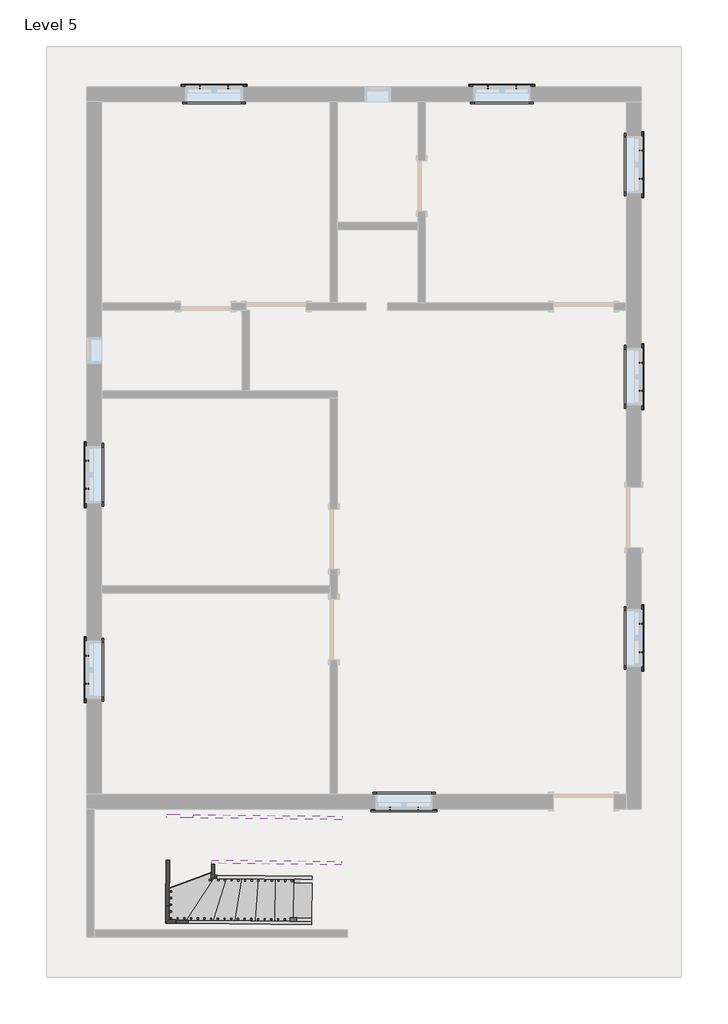
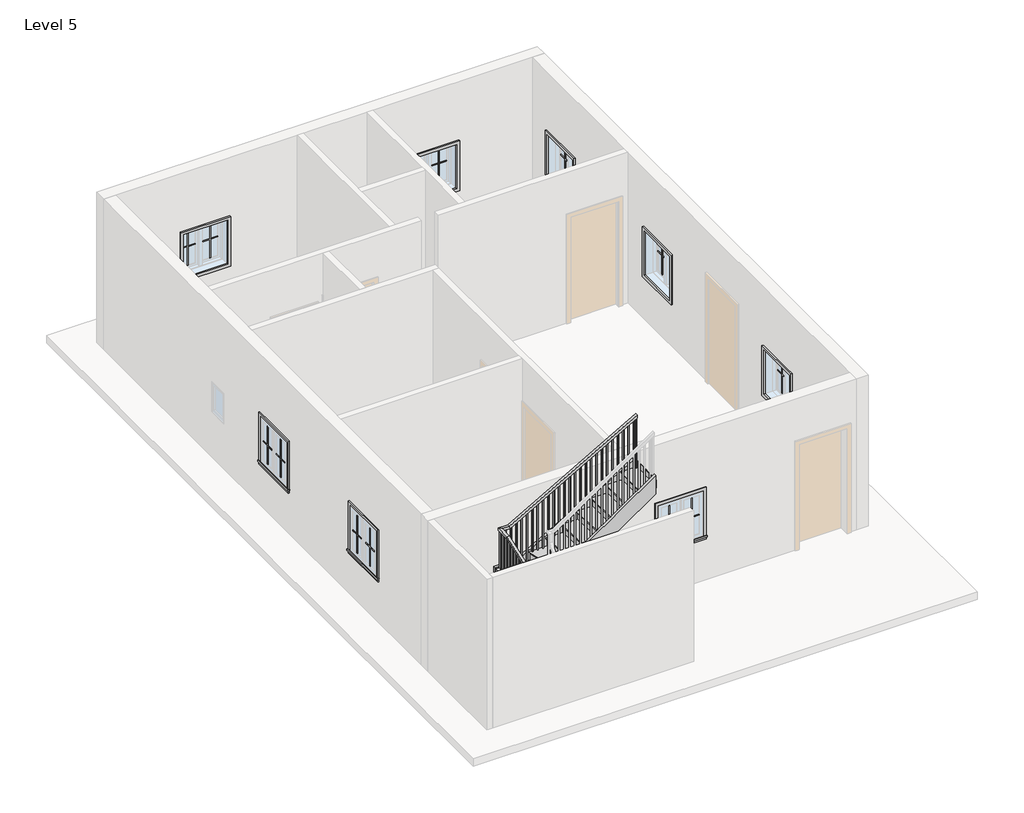
# One storey, part 2 of 2: 32 proxies, 9 members, 1 railing, 1 stair flight.
"""IFC4 building model written with IfcOpenShell, lengths in millimetres."""

from ifc_helpers import new_model, si_unit, frame, origin, place, context, project, spatial, polyline, outline, extrude, faceted_brep, transform, mapped, element, save
from components import muntin_pattern_2x2_muntin_pattern_2x2_b3fe6957, muntin_pattern_2x2_muntin_pattern_2x2_3e0ecaf2, trim_window_exterior_flat_with_sill_41619996, trim_window_interior_flat_picture_frame_51c85655, stair_flight_e36c3716

model = new_model("IFC4")

# Units and contexts
model_context = context("Model", 3, world=origin())
ifc_project = project(units=[si_unit("LENGTHUNIT", "METRE", prefix="MILLI")], contexts=[model_context])

# Site, building, storey
site = spatial("IfcSite", under=ifc_project)
building = spatial("IfcBuilding", under=site)
storey = spatial("IfcBuildingStorey", under=building, Name="Level 5", Elevation=9601.2)

# Proxies
placement = place(None, origin())
muntin_pattern_2x2_muntin_pattern_2x2_shape = muntin_pattern_2x2_muntin_pattern_2x2_b3fe6957(model_context)
element("IfcBuildingElementProxy", 1, Name="Muntin Pattern_2x2 : Muntin Pattern_2x2", ObjectType="Muntin Pattern_2x2 : Muntin Pattern_2x2", at=placement, inside=storey, context=model_context, shape_type="MappedRepresentation", body=[
    mapped(muntin_pattern_2x2_muntin_pattern_2x2_shape, transform((-3662.5622832, 7052.6782079, 10585.45), x_axis=(1.0, 0.0, 0.0), y_axis=(0.0, 1.0, 0.0), z_axis=(0.0, 0.0, 1.0))),
])
element("IfcBuildingElementProxy", 2, Name="Muntin Pattern_2x2 : Muntin Pattern_2x2", ObjectType="Muntin Pattern_2x2 : Muntin Pattern_2x2", at=placement, inside=storey, context=model_context, shape_type="MappedRepresentation", body=[
    mapped(muntin_pattern_2x2_muntin_pattern_2x2_shape, transform((709.4127168, 7052.6782079, 10585.45), x_axis=(1.0, 0.0, 0.0), y_axis=(0.0, 1.0, 0.0), z_axis=(0.0, 0.0, 1.0))),
])
element("IfcBuildingElementProxy", 3, Name="Muntin Pattern_2x2 : Muntin Pattern_2x2", ObjectType="Muntin Pattern_2x2 : Muntin Pattern_2x2", at=placement, inside=storey, context=model_context, shape_type="MappedRepresentation", body=[
    mapped(muntin_pattern_2x2_muntin_pattern_2x2_shape, transform((3028.7502168, 6095.4157079, 10585.45), x_axis=(0.0, -1.0, 0.0), y_axis=(1.0, 0.0, 0.0), z_axis=(0.0, 0.0, 1.0))),
])
element("IfcBuildingElementProxy", 4, Name="Muntin Pattern_2x2 : Muntin Pattern_2x2", ObjectType="Muntin Pattern_2x2 : Muntin Pattern_2x2", at=placement, inside=storey, context=model_context, shape_type="MappedRepresentation", body=[
    mapped(muntin_pattern_2x2_muntin_pattern_2x2_shape, transform((3028.7502168, 2875.9657079, 10585.45), x_axis=(0.0, -1.0, 0.0), y_axis=(1.0, 0.0, 0.0), z_axis=(0.0, 0.0, 1.0))),
])
element("IfcBuildingElementProxy", 5, Name="Muntin Pattern_2x2 : Muntin Pattern_2x2", ObjectType="Muntin Pattern_2x2 : Muntin Pattern_2x2", at=placement, inside=storey, context=model_context, shape_type="MappedRepresentation", body=[
    mapped(muntin_pattern_2x2_muntin_pattern_2x2_shape, transform((3028.7502168, -1086.4342921, 10585.45), x_axis=(0.0, -1.0, 0.0), y_axis=(1.0, 0.0, 0.0), z_axis=(0.0, 0.0, 1.0))),
])
element("IfcBuildingElementProxy", 6, Name="Muntin Pattern_2x2 : Muntin Pattern_2x2", ObjectType="Muntin Pattern_2x2 : Muntin Pattern_2x2", at=placement, inside=storey, context=model_context, shape_type="MappedRepresentation", body=[
    mapped(muntin_pattern_2x2_muntin_pattern_2x2_shape, transform((-5372.2997832, 961.4407079, 10585.45), x_axis=(0.0, 1.0, 0.0), y_axis=(-1.0, 0.0, 0.0), z_axis=(0.0, 0.0, 1.0))),
])
element("IfcBuildingElementProxy", 7, Name="Muntin Pattern_2x2 : Muntin Pattern_2x2", ObjectType="Muntin Pattern_2x2 : Muntin Pattern_2x2", at=placement, inside=storey, context=model_context, shape_type="MappedRepresentation", body=[
    mapped(muntin_pattern_2x2_muntin_pattern_2x2_shape, transform((-5372.2997832, -1997.6592921, 10585.45), x_axis=(0.0, 1.0, 0.0), y_axis=(-1.0, 0.0, 0.0), z_axis=(0.0, 0.0, 1.0))),
])
element("IfcBuildingElementProxy", 8, Name="Muntin Pattern_2x2 : Muntin Pattern_2x2", ObjectType="Muntin Pattern_2x2 : Muntin Pattern_2x2", at=placement, inside=storey, context=model_context, shape_type="MappedRepresentation", body=[
    mapped(muntin_pattern_2x2_muntin_pattern_2x2_shape, transform((-347.8622832, -3888.3717921, 10585.45), x_axis=(-1.0, 0.0, 0.0), y_axis=(0.0, -1.0, 0.0), z_axis=(0.0, 0.0, 1.0))),
])
muntin_pattern_2x2_muntin_pattern_2x2_2_shape = muntin_pattern_2x2_muntin_pattern_2x2_3e0ecaf2(model_context)
element("IfcBuildingElementProxy", 9, Name="Muntin Pattern_2x2 : Muntin Pattern_2x2", ObjectType="Muntin Pattern_2x2 : Muntin Pattern_2x2", at=placement, inside=storey, context=model_context, shape_type="MappedRepresentation", body=[
    mapped(muntin_pattern_2x2_muntin_pattern_2x2_2_shape, transform((-3233.9372832, 7052.6782079, 10585.45), x_axis=(-1.0, 0.0, 0.0), y_axis=(0.0, -1.0, 0.0), z_axis=(0.0, 0.0, 1.0))),
])
element("IfcBuildingElementProxy", 10, Name="Muntin Pattern_2x2 : Muntin Pattern_2x2", ObjectType="Muntin Pattern_2x2 : Muntin Pattern_2x2", at=placement, inside=storey, context=model_context, shape_type="MappedRepresentation", body=[
    mapped(muntin_pattern_2x2_muntin_pattern_2x2_2_shape, transform((1138.0377168, 7052.6782079, 10585.45), x_axis=(-1.0, 0.0, 0.0), y_axis=(0.0, -1.0, 0.0), z_axis=(0.0, 0.0, 1.0))),
])
element("IfcBuildingElementProxy", 11, Name="Muntin Pattern_2x2 : Muntin Pattern_2x2", ObjectType="Muntin Pattern_2x2 : Muntin Pattern_2x2", at=placement, inside=storey, context=model_context, shape_type="MappedRepresentation", body=[
    mapped(muntin_pattern_2x2_muntin_pattern_2x2_2_shape, transform((3028.7502168, 5666.7907079, 10585.45), x_axis=(0.0, 1.0, 0.0), y_axis=(-1.0, 0.0, 0.0), z_axis=(0.0, 0.0, 1.0))),
])
element("IfcBuildingElementProxy", 12, Name="Muntin Pattern_2x2 : Muntin Pattern_2x2", ObjectType="Muntin Pattern_2x2 : Muntin Pattern_2x2", at=placement, inside=storey, context=model_context, shape_type="MappedRepresentation", body=[
    mapped(muntin_pattern_2x2_muntin_pattern_2x2_2_shape, transform((3028.7502168, 2447.3407079, 10585.45), x_axis=(0.0, 1.0, 0.0), y_axis=(-1.0, 0.0, 0.0), z_axis=(0.0, 0.0, 1.0))),
])
element("IfcBuildingElementProxy", 13, Name="Muntin Pattern_2x2 : Muntin Pattern_2x2", ObjectType="Muntin Pattern_2x2 : Muntin Pattern_2x2", at=placement, inside=storey, context=model_context, shape_type="MappedRepresentation", body=[
    mapped(muntin_pattern_2x2_muntin_pattern_2x2_2_shape, transform((3028.7502168, -1515.0592921, 10585.45), x_axis=(0.0, 1.0, 0.0), y_axis=(-1.0, 0.0, 0.0), z_axis=(0.0, 0.0, 1.0))),
])
element("IfcBuildingElementProxy", 14, Name="Muntin Pattern_2x2 : Muntin Pattern_2x2", ObjectType="Muntin Pattern_2x2 : Muntin Pattern_2x2", at=placement, inside=storey, context=model_context, shape_type="MappedRepresentation", body=[
    mapped(muntin_pattern_2x2_muntin_pattern_2x2_2_shape, transform((-5372.2997832, 1390.0657079, 10585.45), x_axis=(0.0, -1.0, 0.0), y_axis=(1.0, 0.0, 0.0), z_axis=(0.0, 0.0, 1.0))),
])
element("IfcBuildingElementProxy", 15, Name="Muntin Pattern_2x2 : Muntin Pattern_2x2", ObjectType="Muntin Pattern_2x2 : Muntin Pattern_2x2", at=placement, inside=storey, context=model_context, shape_type="MappedRepresentation", body=[
    mapped(muntin_pattern_2x2_muntin_pattern_2x2_2_shape, transform((-5372.2997832, -1569.0342921, 10585.45), x_axis=(0.0, -1.0, 0.0), y_axis=(1.0, 0.0, 0.0), z_axis=(0.0, 0.0, 1.0))),
])
element("IfcBuildingElementProxy", 16, Name="Muntin Pattern_2x2 : Muntin Pattern_2x2", ObjectType="Muntin Pattern_2x2 : Muntin Pattern_2x2", at=placement, inside=storey, context=model_context, shape_type="MappedRepresentation", body=[
    mapped(muntin_pattern_2x2_muntin_pattern_2x2_2_shape, transform((-776.4872832, -3888.3717921, 10585.45), x_axis=(1.0, 0.0, 0.0), y_axis=(0.0, 1.0, 0.0), z_axis=(0.0, 0.0, 1.0))),
])
trim_window_exterior_flat_with_sill_shape = trim_window_exterior_flat_with_sill_41619996(model_context)
element("IfcBuildingElementProxy", 17, Name="Trim-Window-Exterior-Flat : with Sill", ObjectType="Trim-Window-Exterior-Flat : with Sill", at=placement, inside=storey, context=model_context, shape_type="MappedRepresentation", body=[
    mapped(trim_window_exterior_flat_with_sill_shape, transform((-3448.2497832, 7062.2032079, 11430.0), x_axis=(-1.0, 0.0, 0.0), y_axis=(0.0, 0.0, 1.0), z_axis=(0.0, 1.0, 0.0))),
])
element("IfcBuildingElementProxy", 18, Name="Trim-Window-Exterior-Flat : with Sill", ObjectType="Trim-Window-Exterior-Flat : with Sill", at=placement, inside=storey, context=model_context, shape_type="MappedRepresentation", body=[
    mapped(trim_window_exterior_flat_with_sill_shape, transform((923.7252168, 7062.2032079, 11430.0), x_axis=(-1.0, 0.0, 0.0), y_axis=(0.0, 0.0, 1.0), z_axis=(0.0, 1.0, 0.0))),
])
element("IfcBuildingElementProxy", 19, Name="Trim-Window-Exterior-Flat : with Sill", ObjectType="Trim-Window-Exterior-Flat : with Sill", at=placement, inside=storey, context=model_context, shape_type="MappedRepresentation", body=[
    mapped(trim_window_exterior_flat_with_sill_shape, transform((3038.2752168, 5881.1032079, 11430.0), x_axis=(0.0, 1.0, 0.0), y_axis=(0.0, 0.0, 1.0), z_axis=(1.0, 0.0, 0.0))),
])
element("IfcBuildingElementProxy", 20, Name="Trim-Window-Exterior-Flat : with Sill", ObjectType="Trim-Window-Exterior-Flat : with Sill", at=placement, inside=storey, context=model_context, shape_type="MappedRepresentation", body=[
    mapped(trim_window_exterior_flat_with_sill_shape, transform((3038.2752168, 2661.6532079, 11430.0), x_axis=(0.0, 1.0, 0.0), y_axis=(0.0, 0.0, 1.0), z_axis=(1.0, 0.0, 0.0))),
])
element("IfcBuildingElementProxy", 21, Name="Trim-Window-Exterior-Flat : with Sill", ObjectType="Trim-Window-Exterior-Flat : with Sill", at=placement, inside=storey, context=model_context, shape_type="MappedRepresentation", body=[
    mapped(trim_window_exterior_flat_with_sill_shape, transform((3038.2752168, -1300.7467921, 11430.0), x_axis=(0.0, 1.0, 0.0), y_axis=(0.0, 0.0, 1.0), z_axis=(1.0, 0.0, 0.0))),
])
element("IfcBuildingElementProxy", 22, Name="Trim-Window-Exterior-Flat : with Sill", ObjectType="Trim-Window-Exterior-Flat : with Sill", at=placement, inside=storey, context=model_context, shape_type="MappedRepresentation", body=[
    mapped(trim_window_exterior_flat_with_sill_shape, transform((-5381.8247832, 1175.7532079, 11430.0), x_axis=(0.0, -1.0, 0.0), y_axis=(0.0, 0.0, 1.0), z_axis=(-1.0, 0.0, 0.0))),
])
element("IfcBuildingElementProxy", 23, Name="Trim-Window-Exterior-Flat : with Sill", ObjectType="Trim-Window-Exterior-Flat : with Sill", at=placement, inside=storey, context=model_context, shape_type="MappedRepresentation", body=[
    mapped(trim_window_exterior_flat_with_sill_shape, transform((-5381.8247832, -1783.3467921, 11430.0), x_axis=(0.0, -1.0, 0.0), y_axis=(0.0, 0.0, 1.0), z_axis=(-1.0, 0.0, 0.0))),
])
element("IfcBuildingElementProxy", 24, Name="Trim-Window-Exterior-Flat : with Sill", ObjectType="Trim-Window-Exterior-Flat : with Sill", at=placement, inside=storey, context=model_context, shape_type="MappedRepresentation", body=[
    mapped(trim_window_exterior_flat_with_sill_shape, transform((-562.1747832, -3897.8967921, 11430.0), x_axis=(1.0, 0.0, 0.0), y_axis=(0.0, 0.0, 1.0), z_axis=(0.0, -1.0, 0.0))),
])
trim_window_interior_flat_picture_frame_shape = trim_window_interior_flat_picture_frame_51c85655(model_context)
element("IfcBuildingElementProxy", 25, Name="Trim-Window-Interior-Flat : Picture Frame", ObjectType="Trim-Window-Interior-Flat : Picture Frame", at=placement, inside=storey, context=model_context, shape_type="MappedRepresentation", body=[
    mapped(trim_window_interior_flat_picture_frame_shape, transform((-3448.2497832, 6833.6032079, 11430.0), x_axis=(1.0, 0.0, 0.0), y_axis=(0.0, 0.0, 1.0), z_axis=(0.0, -1.0, 0.0))),
])
element("IfcBuildingElementProxy", 26, Name="Trim-Window-Interior-Flat : Picture Frame", ObjectType="Trim-Window-Interior-Flat : Picture Frame", at=placement, inside=storey, context=model_context, shape_type="MappedRepresentation", body=[
    mapped(trim_window_interior_flat_picture_frame_shape, transform((923.7252168, 6833.6032079, 11430.0), x_axis=(1.0, 0.0, 0.0), y_axis=(0.0, 0.0, 1.0), z_axis=(0.0, -1.0, 0.0))),
])
element("IfcBuildingElementProxy", 27, Name="Trim-Window-Interior-Flat : Picture Frame", ObjectType="Trim-Window-Interior-Flat : Picture Frame", at=placement, inside=storey, context=model_context, shape_type="MappedRepresentation", body=[
    mapped(trim_window_interior_flat_picture_frame_shape, transform((2809.6752168, 5881.1032079, 11430.0), x_axis=(0.0, -1.0, 0.0), y_axis=(0.0, 0.0, 1.0), z_axis=(-1.0, 0.0, 0.0))),
])
element("IfcBuildingElementProxy", 28, Name="Trim-Window-Interior-Flat : Picture Frame", ObjectType="Trim-Window-Interior-Flat : Picture Frame", at=placement, inside=storey, context=model_context, shape_type="MappedRepresentation", body=[
    mapped(trim_window_interior_flat_picture_frame_shape, transform((2809.6752168, 2661.6532079, 11430.0), x_axis=(0.0, -1.0, 0.0), y_axis=(0.0, 0.0, 1.0), z_axis=(-1.0, 0.0, 0.0))),
])
element("IfcBuildingElementProxy", 29, Name="Trim-Window-Interior-Flat : Picture Frame", ObjectType="Trim-Window-Interior-Flat : Picture Frame", at=placement, inside=storey, context=model_context, shape_type="MappedRepresentation", body=[
    mapped(trim_window_interior_flat_picture_frame_shape, transform((2809.6752168, -1300.7467921, 11430.0), x_axis=(0.0, -1.0, 0.0), y_axis=(0.0, 0.0, 1.0), z_axis=(-1.0, 0.0, 0.0))),
])
element("IfcBuildingElementProxy", 30, Name="Trim-Window-Interior-Flat : Picture Frame", ObjectType="Trim-Window-Interior-Flat : Picture Frame", at=placement, inside=storey, context=model_context, shape_type="MappedRepresentation", body=[
    mapped(trim_window_interior_flat_picture_frame_shape, transform((-5153.2247832, 1175.7532079, 11430.0), x_axis=(0.0, 1.0, 0.0), y_axis=(0.0, 0.0, 1.0), z_axis=(1.0, 0.0, 0.0))),
])
element("IfcBuildingElementProxy", 31, Name="Trim-Window-Interior-Flat : Picture Frame", ObjectType="Trim-Window-Interior-Flat : Picture Frame", at=placement, inside=storey, context=model_context, shape_type="MappedRepresentation", body=[
    mapped(trim_window_interior_flat_picture_frame_shape, transform((-5153.2247832, -1783.3467921, 11430.0), x_axis=(0.0, 1.0, 0.0), y_axis=(0.0, 0.0, 1.0), z_axis=(1.0, 0.0, 0.0))),
])
element("IfcBuildingElementProxy", 32, Name="Trim-Window-Interior-Flat : Picture Frame", ObjectType="Trim-Window-Interior-Flat : Picture Frame", at=placement, inside=storey, context=model_context, shape_type="MappedRepresentation", body=[
    mapped(trim_window_interior_flat_picture_frame_shape, transform((-562.1747832, -3669.2967921, 11430.0), x_axis=(-1.0, 0.0, 0.0), y_axis=(0.0, 0.0, 1.0), z_axis=(0.0, 1.0, 0.0))),
])

# Members
element("IfcMember", 33, ObjectType="Stringer - 2\" Width", at=placement, inside=storey, context=model_context, shape_type="SweptSolid", body=[
    extrude(outline(polyline([(-105.6395382, -202.4353776), (0.0, 0.0), (2328.2458671, 0.0), (2169.1880402, -304.8), (90.52017, -304.8), (-105.6395382, -202.4353776)])), frame((-1968.9977307, -5651.1672049, 9829.5413982), z_axis=(0.01073603161956521, 0.9999423671517593, 0.0), x_axis=(-0.8864958884204138, 0.009517996437940355, 0.46263857119517027)), (0.0, 0.0, 1.0), 50.8),
])
element("IfcMember", 34, ObjectType="Stringer - 2\" Width", at=placement, inside=storey, context=model_context, shape_type="SweptSolid", body=[
    extrude(outline(polyline([(-4032.4327287, -5578.2098967), (-4032.9781191, -5629.006969), (-4182.4018504, -5627.4026586), (-4131.0593878, -5577.1509768), (-4032.4327287, -5578.2098967)])), frame((0.0, 0.0, 10562.8719334), z_axis=(0.0, 0.0, 1.0), x_axis=(1.0, 0.0, 0.0)), (0.0, 0.0, 1.0), 343.8058061),
])
element("IfcMember", 35, ObjectType="Stringer - 2\" Width", at=placement, inside=storey, context=model_context, shape_type="SweptSolid", body=[
    extrude(outline(polyline([(-4131.0593878, -5577.1509768), (-4182.4018504, -5627.4026586), (-4179.6442274, -5370.5606366), (-4128.8471552, -5371.106027), (-4131.0593878, -5577.1509768)])), frame((0.0, 0.0, 10562.8719334), z_axis=(0.0, 0.0, 1.0), x_axis=(1.0, 0.0, 0.0)), (0.0, 0.0, 1.0), 343.8058061),
])
element("IfcMember", 36, ObjectType="Stringer - 2\" Width", at=placement, inside=storey, context=model_context, shape_type="SweptSolid", body=[
    extrude(outline(polyline([(110.9788635, -325.4014815), (0.0, 0.0), (1419.3210826, 0.0), (1526.5904374, -314.5248191), (1494.6989405, -325.4014816), (110.9788635, -325.4014815)])), frame((-4128.8471552, -5371.106027, 10562.8719334), z_axis=(-0.9999423671517593, 0.010736031619565298, 0.0), x_axis=(0.010161319362697869, 0.946414289466532, 0.3227951986668461)), (0.0, 0.0, 1.0), 50.8),
])
element("IfcMember", 37, ObjectType="Stringer - 2\" Width", at=placement, inside=storey, context=model_context, shape_type="SweptSolid", body=[
    extrude(outline(polyline([(-4165.2220526, -4027.2948827), (-4164.6766622, -3976.4978105), (-3763.6581151, -3980.8034064), (-3764.2035055, -4031.6004787), (-4165.2220526, -4027.2948827)])), frame((0.0, 0.0, 11031.2968076), z_axis=(0.0, 0.0, 1.0), x_axis=(1.0, 0.0, 0.0)), (0.0, 0.0, 1.0), 322.0391291),
])
element("IfcMember", 38, ObjectType="Stringer - 2\" Width", at=placement, inside=storey, context=model_context, shape_type="SweptSolid", body=[
    extrude(outline(polyline([(-111.9640108, -160.4153284), (0.0, 0.0), (1801.1015507, 0.0), (1588.362339, -304.8), (94.9016984, -304.8), (-111.9640108, -160.4153284)])), frame((-1961.6349602, -4965.4067295, 9796.8246848), z_axis=(0.010736031619565371, 0.9999423671517593, 0.0), x_axis=(-0.8199685195580257, 0.008803715336213096, 0.5723409137307053)), (0.0, 0.0, 1.0), 50.8),
])
element("IfcMember", 39, ObjectType="Stringer - 2\" Width", at=placement, inside=storey, context=model_context, shape_type="SweptSolid", body=[
    extrude(outline(polyline([(451.3522078, -304.8), (7.554265, -5.1014262), (10.999279, 0.0), (408.4725128, 0.0), (831.8908901, -285.9361695), (819.1520678, -304.8), (451.3522078, -304.8)])), frame((-3438.4815323, -4949.5503441, 10482.3097108), z_axis=(-0.9999423671517593, 0.010736031619565902, 0.0), x_axis=(0.00600837694393381, 0.559613726649973, 0.8287317879455506)), (0.0, 0.0, 1.0), 50.8),
])
element("IfcMember", 40, ObjectType="Stringer - 2\" Width", at=placement, inside=storey, context=model_context, shape_type="SweptSolid", body=[
    extrude(outline(polyline([(215.732707, -304.8), (0.0, 0.0), (2421.4097535, 0.0), (2637.1424605, -304.8), (215.732707, -304.8)])), frame((-3486.8243477, -4720.4181286, 10958.3256311), z_axis=(0.010736031619565212, 0.9999423671517593, 0.0), x_axis=(0.8161886957592971, -0.008763132689499912, 0.5777189804915569)), (0.0, 0.0, 1.0), 50.8),
])
element("IfcMember", 41, ObjectType="Stringer - 2\" Width", at=placement, inside=storey, context=model_context, shape_type="SweptSolid", body=[
    extrude(outline(polyline([(161.6856691, -278.5084291), (0.0, 0.0), (2614.6236412, 0.0), (2776.3093103, -278.508429), (161.6856691, -278.5084291)])), frame((-3764.2035055, -4031.6004787, 11031.2968076), z_axis=(0.01073603161956531, 0.9999423671517593, 0.0), x_axis=(0.8647780740833296, -0.009284819857879231, 0.5020683964410966)), (0.0, 0.0, 1.0), 50.8),
])

# Railing
element("IfcRailing", 42, ObjectType="Handrail - Rectangular", at=placement, inside=storey, context=model_context, shape_type="SolidModel", body=[
    faceted_brep([(-1968.4523403, -5600.3701326, 10684.9333333), (-1968.4523403, -5600.3701326, 10627.3388957), (-1967.9069499, -5549.5730604, 10627.3388957), (-1967.9069499, -5549.5730604, 10684.9333333), (-4009.5042766, -5578.4560715, 11775.3579081), (-4022.2220752, -5578.319525, 11724.5579081), (-4021.6766848, -5527.5224527, 11724.5579081), (-4008.9588862, -5527.6589993, 11775.3579081), (-4131.0593878, -5577.1509768, 11775.3579081), (-4131.0593878, -5577.1509768, 11724.5579081), (-4079.7169251, -5526.8992949, 11724.5579081), (-4079.7169251, -5526.8992949, 11775.3579081), (-4129.1695675, -5401.1351667, 11775.3579081), (-4129.079122, -5392.7111679, 11724.5579081), (-4078.2820498, -5393.2565584, 11724.5579081), (-4078.3724953, -5401.6805571, 11775.3579081), (-4117.5603361, -4319.8639155, 12144.1490097), (-4117.4698906, -4311.4399167, 12093.3490097), (-4066.6728183, -4311.9853071, 12093.3490097), (-4066.7632639, -4320.4093059, 12144.1490097), (-4114.4249804, -4027.8402731, 12144.1490097), (-4114.4249804, -4027.8402731, 12093.3490097), (-4064.1732985, -4079.1827358, 12093.3490097), (-4064.1732985, -4079.1827358, 12144.1490097), (-3933.3337165, -4029.7845867, 12144.1490097), (-3919.5861077, -4029.93219, 12093.3490097), (-3920.1314981, -4080.7292622, 12093.3490097), (-3933.8791069, -4080.581659, 12144.1490097), (-1503.1343086, -4055.8767882, 13563.6), (-1503.679699, -4106.6738604, 13563.6), (-1503.679699, -4106.6738604, 13504.7701828), (-1503.1343086, -4055.8767882, 13504.7701828)], [[[0, 1, 2, 3]], [[1, 0, 4, 5]], [[2, 1, 5, 6]], [[3, 2, 6, 7]], [[0, 3, 7, 4]], [[5, 4, 8, 9]], [[6, 5, 9, 10]], [[7, 6, 10, 11]], [[4, 7, 11, 8]], [[9, 8, 12, 13]], [[10, 9, 13, 14]], [[11, 10, 14, 15]], [[8, 11, 15, 12]], [[13, 12, 16, 17]], [[14, 13, 17, 18]], [[15, 14, 18, 19]], [[12, 15, 19, 16]], [[17, 16, 20, 21]], [[18, 17, 21, 22]], [[19, 18, 22, 23]], [[16, 19, 23, 20]], [[21, 20, 24, 25]], [[22, 21, 25, 26]], [[23, 22, 26, 27]], [[20, 23, 27, 24]], [[28, 29, 30, 31]], [[25, 24, 28, 31]], [[26, 25, 31, 30]], [[27, 26, 30, 29]], [[24, 27, 29, 28]]]),
    extrude(outline(polyline([(234.1631202, 19.05), (1226.6129544, 19.05), (1226.6129544, 0.0), (223.0368797, 0.0), (234.1631202, 19.05)])), frame((-1540.0233365, -4090.4077365, 13706.4796211), z_axis=(0.010736031619565153, 0.9999423671517594, 0.0), x_axis=(0.0, 0.0, -1.0)), (0.0, 0.0, 1.0), 19.05),
    extrude(outline(polyline([(234.1631202, 19.05), (1167.2730054, 19.05), (1167.2730054, 0.0), (223.0368798, 0.0), (234.1631202, 19.05)])), frame((-1641.617481, -4089.3169557, 13647.1396721), z_axis=(0.010736031619565153, 0.9999423671517594, 0.0), x_axis=(0.0, 0.0, -1.0)), (0.0, 0.0, 1.0), 19.05),
    extrude(outline(polyline([(234.1631202, 19.05), (1107.9330563, 19.05), (1107.9330563, 0.0), (223.0368797, 0.0), (234.1631202, 19.05)])), frame((-1743.2116255, -4088.2261749, 13587.799723), z_axis=(0.010736031619565153, 0.9999423671517594, 0.0), x_axis=(0.0, 0.0, -1.0)), (0.0, 0.0, 1.0), 19.05),
    extrude(outline(polyline([(234.1631202, 19.05), (1217.9264407, 19.05), (1217.9264407, 0.0), (223.0368798, 0.0), (234.1631202, 19.05)])), frame((-1844.80577, -4087.1353941, 13528.459774), z_axis=(0.010736031619565153, 0.9999423671517594, 0.0), x_axis=(0.0, 0.0, -1.0)), (0.0, 0.0, 1.0), 19.05),
    extrude(outline(polyline([(234.1631203, 19.05), (1158.5864917, 19.05), (1158.5864917, 0.0), (223.0368798, 0.0), (234.1631203, 19.05)])), frame((-1946.3999145, -4086.0446133, 13469.119825), z_axis=(0.010736031619565153, 0.9999423671517594, 0.0), x_axis=(0.0, 0.0, -1.0)), (0.0, 0.0, 1.0), 19.05),
    extrude(outline(polyline([(234.1631202, 19.05), (1099.2465426, 19.05), (1099.2465426, 0.0), (223.0368798, 0.0), (234.1631202, 19.05)])), frame((-2047.994059, -4084.9538324, 13409.7798759), z_axis=(0.010736031619565153, 0.9999423671517594, 0.0), x_axis=(0.0, 0.0, -1.0)), (0.0, 0.0, 1.0), 19.05),
    extrude(outline(polyline([(234.1631202, 19.0499999), (1209.2399269, 19.0499999), (1209.2399269, 0.0), (223.0368798, 0.0), (234.1631202, 19.0499999)])), frame((-2149.5882036, -4083.8630516, 13350.4399269), z_axis=(0.010736031619565153, 0.9999423671517594, 0.0), x_axis=(0.0, 0.0, -1.0)), (0.0, 0.0, 1.0), 19.05),
    extrude(outline(polyline([(234.1631202, 19.0499999), (1149.8999778, 19.0499999), (1149.8999778, 0.0), (223.0368797, 0.0), (234.1631202, 19.0499999)])), frame((-2251.1823481, -4082.7722708, 13291.0999778), z_axis=(0.010736031619565153, 0.9999423671517594, 0.0), x_axis=(0.0, 0.0, -1.0)), (0.0, 0.0, 1.0), 19.05),
    extrude(outline(polyline([(234.1631202, 19.05), (1259.8933621, 19.05), (1259.8933621, 0.0), (223.0368798, 0.0), (234.1631202, 19.05)])), frame((-2352.7764926, -4081.68149, 13231.7600288), z_axis=(0.010736031619565153, 0.9999423671517594, 0.0), x_axis=(0.0, 0.0, -1.0)), (0.0, 0.0, 1.0), 19.05),
    extrude(outline(polyline([(234.1631203, 19.05), (1200.5534131, 19.05), (1200.5534131, 0.0), (223.0368798, 0.0), (234.1631203, 19.05)])), frame((-2454.3706371, -4080.5907092, 13172.4200798), z_axis=(0.010736031619565153, 0.9999423671517594, 0.0), x_axis=(0.0, 0.0, -1.0)), (0.0, 0.0, 1.0), 19.05),
    extrude(outline(polyline([(234.1631202, 19.05), (1141.213464, 19.05), (1141.213464, 0.0), (223.0368798, 0.0), (234.1631202, 19.05)])), frame((-2555.9647816, -4079.4999284, 13113.0801307), z_axis=(0.010736031619565153, 0.9999423671517594, 0.0), x_axis=(0.0, 0.0, -1.0)), (0.0, 0.0, 1.0), 19.05),
    extrude(outline(polyline([(234.1631203, 19.05), (1251.2068484, 19.05), (1251.2068484, 0.0), (223.0368798, 0.0), (234.1631203, 19.05)])), frame((-2657.5589261, -4078.4091476, 13053.7401817), z_axis=(0.010736031619565153, 0.9999423671517594, 0.0), x_axis=(0.0, 0.0, -1.0)), (0.0, 0.0, 1.0), 19.05),
    extrude(outline(polyline([(234.1631202, 19.05), (1191.8668993, 19.05), (1191.8668993, 0.0), (223.0368797, 0.0), (234.1631202, 19.05)])), frame((-2759.1530706, -4077.3183668, 12994.4002326), z_axis=(0.010736031619565153, 0.9999423671517594, 0.0), x_axis=(0.0, 0.0, -1.0)), (0.0, 0.0, 1.0), 19.05),
    extrude(outline(polyline([(234.1631202, 19.05), (1132.5269503, 19.05), (1132.5269503, 0.0), (223.0368798, 0.0), (234.1631202, 19.05)])), frame((-2860.7472151, -4076.2275859, 12935.0602836), z_axis=(0.010736031619565153, 0.9999423671517594, 0.0), x_axis=(0.0, 0.0, -1.0)), (0.0, 0.0, 1.0), 19.05),
    extrude(outline(polyline([(234.1631202, 19.05), (1242.5203345, 19.05), (1242.5203345, 0.0), (223.0368797, 0.0), (234.1631202, 19.05)])), frame((-2962.3413596, -4075.1368051, 12875.7203345), z_axis=(0.010736031619565153, 0.9999423671517594, 0.0), x_axis=(0.0, 0.0, -1.0)), (0.0, 0.0, 1.0), 19.05),
    extrude(outline(polyline([(234.1631202, 19.05), (1183.1803855, 19.05), (1183.1803855, 0.0), (223.0368798, 0.0), (234.1631202, 19.05)])), frame((-3063.9355041, -4074.0460243, 12816.3803855), z_axis=(0.010736031619565153, 0.9999423671517594, 0.0), x_axis=(0.0, 0.0, -1.0)), (0.0, 0.0, 1.0), 19.05),
    extrude(outline(polyline([(234.1631203, 19.05), (1123.8404365, 19.05), (1123.8404365, 0.0), (223.0368798, 0.0), (234.1631203, 19.05)])), frame((-3165.5296486, -4072.9552435, 12757.0404365), z_axis=(0.010736031619565153, 0.9999423671517594, 0.0), x_axis=(0.0, 0.0, -1.0)), (0.0, 0.0, 1.0), 19.05),
    extrude(outline(polyline([(234.1631202, 19.05), (1233.8338207, 19.05), (1233.8338207, 0.0), (223.0368798, 0.0), (234.1631202, 19.05)])), frame((-3267.1237931, -4071.8644627, 12697.7004874), z_axis=(0.010736031619565153, 0.9999423671517594, 0.0), x_axis=(0.0, 0.0, -1.0)), (0.0, 0.0, 1.0), 19.05),
    extrude(outline(polyline([(234.1631202, 19.05), (1174.4938717, 19.05), (1174.4938717, 0.0), (223.0368798, 0.0), (234.1631202, 19.05)])), frame((-3368.7179376, -4070.7736819, 12638.3605384), z_axis=(0.010736031619565153, 0.9999423671517594, 0.0), x_axis=(0.0, 0.0, -1.0)), (0.0, 0.0, 1.0), 19.05),
    extrude(outline(polyline([(234.1631202, 19.05), (1115.1539226, 19.05), (1115.1539226, 0.0), (223.0368797, 0.0), (234.1631202, 19.05)])), frame((-3470.3120821, -4069.6829011, 12579.0205893), z_axis=(0.010736031619565153, 0.9999423671517594, 0.0), x_axis=(0.0, 0.0, -1.0)), (0.0, 0.0, 1.0), 19.05),
    extrude(outline(polyline([(234.1631202, 19.05), (1225.147307, 19.05), (1225.147307, 0.0), (223.0368798, 0.0), (234.1631202, 19.05)])), frame((-3571.9062266, -4068.5921203, 12519.6806403), z_axis=(0.010736031619565153, 0.9999423671517594, 0.0), x_axis=(0.0, 0.0, -1.0)), (0.0, 0.0, 1.0), 19.05),
    extrude(outline(polyline([(234.1631202, 19.05), (1165.8073579, 19.05), (1165.8073579, 0.0), (223.0368797, 0.0), (234.1631202, 19.05)])), frame((-3673.5003711, -4067.5013394, 12460.3406912), z_axis=(0.010736031619565153, 0.9999423671517594, 0.0), x_axis=(0.0, 0.0, -1.0)), (0.0, 0.0, 1.0), 19.05),
    extrude(outline(polyline([(234.1631202, 19.05), (1106.4674089, 19.05), (1106.4674089, 0.0), (223.0368798, 0.0), (234.1631202, 19.05)])), frame((-3775.0945156, -4066.4105586, 12401.0007422), z_axis=(0.010736031619565153, 0.9999423671517594, 0.0), x_axis=(0.0, 0.0, -1.0)), (0.0, 0.0, 1.0), 19.05),
    extrude(outline(polyline([(234.1631203, 19.05), (1047.1274599, 19.05), (1047.1274599, 0.0), (223.0368798, 0.0), (234.1631203, 19.05)])), frame((-3876.6886601, -4065.3197778, 12341.6607932), z_axis=(0.010736031619565153, 0.9999423671517594, 0.0), x_axis=(0.0, 0.0, -1.0)), (0.0, 0.0, 1.0), 19.05),
    extrude(outline(polyline([(-3997.1271853, -4044.9755735), (-3978.0782832, -4045.1800949), (-3978.2828046, -4064.228997), (-3997.3317067, -4064.0244756), (-3997.1271853, -4044.9755735)])), frame((0.0, 0.0, 11294.5333333), z_axis=(0.0, 0.0, 1.0), x_axis=(1.0, 0.0, 0.0)), (0.0, 0.0, 1.0), 798.8156763),
    extrude(outline(polyline([(-4099.7439368, -4139.1293032), (-4099.5394154, -4120.0804011), (-4080.4905133, -4120.2849225), (-4080.6950347, -4139.3338246), (-4099.7439368, -4139.1293032)])), frame((0.0, 0.0, 11294.5333333), z_axis=(0.0, 0.0, 1.0), x_axis=(1.0, 0.0, 0.0)), (0.0, 0.0, 1.0), 798.8156763),
    extrude(outline(polyline([(-4100.8347176, -4240.7234477), (-4100.6301962, -4221.6745456), (-4081.5812941, -4221.879067), (-4081.7858155, -4240.9279691), (-4100.8347176, -4240.7234477)])), frame((0.0, 0.0, 11125.2), z_axis=(0.0, 0.0, 1.0), x_axis=(1.0, 0.0, 0.0)), (0.0, 0.0, 1.0), 968.1490097),
    extrude(outline(polyline([(231.8485214, 19.05), (1189.524158, 19.05), (1189.524158, 0.0), (225.3514786, 0.0), (231.8485214, 19.05)])), frame((-4082.6720749, -4323.4732115, 12314.724158), z_axis=(-0.9999423671517593, 0.010736031619565137, 0.0), x_axis=(0.0, 0.0, -1.0)), (0.0, 0.0, 1.0), 19.05),
    extrude(outline(polyline([(231.8485214, 19.05), (1154.8732631, 19.05), (1154.8732631, 0.0), (225.3514786, 0.0), (231.8485214, 19.05)])), frame((-4083.7628557, -4425.067356, 12280.0732631), z_axis=(-0.9999423671517593, 0.010736031619565137, 0.0), x_axis=(0.0, 0.0, -1.0)), (0.0, 0.0, 1.0), 19.05),
    extrude(outline(polyline([(231.8485214, 19.05), (1120.2223682, 19.05), (1120.2223682, 0.0), (225.3514786, 0.0), (231.8485214, 19.05)])), frame((-4084.8536366, -4526.6615005, 12245.4223682), z_axis=(-0.9999423671517593, 0.010736031619565137, 0.0), x_axis=(0.0, 0.0, -1.0)), (0.0, 0.0, 1.0), 19.05),
    extrude(outline(polyline([(231.8485214, 19.05), (1085.5714733, 19.05), (1085.5714733, 0.0), (225.3514786, 0.0), (231.8485214, 19.05)])), frame((-4085.9444174, -4628.255645, 12210.7714733), z_axis=(-0.9999423671517593, 0.010736031619565137, 0.0), x_axis=(0.0, 0.0, -1.0)), (0.0, 0.0, 1.0), 19.05),
    extrude(outline(polyline([(231.8485214, 19.05), (1220.2539118, 19.05), (1220.2539118, 0.0), (225.3514786, 0.0), (231.8485214, 19.05)])), frame((-4087.0351982, -4729.8497895, 12176.1205785), z_axis=(-0.9999423671517593, 0.010736031619565137, 0.0), x_axis=(0.0, 0.0, -1.0)), (0.0, 0.0, 1.0), 19.05),
    extrude(outline(polyline([(231.8485214, 19.05), (1185.6030169, 19.05), (1185.6030169, 0.0), (225.3514786, 0.0), (231.8485214, 19.05)])), frame((-4088.125979, -4831.443934, 12141.4696836), z_axis=(-0.9999423671517593, 0.010736031619565137, 0.0), x_axis=(0.0, 0.0, -1.0)), (0.0, 0.0, 1.0), 19.05),
    extrude(outline(polyline([(231.8485214, 19.05), (1150.952122, 19.05), (1150.952122, 0.0), (225.3514786, 0.0), (231.8485214, 19.05)])), frame((-4089.2167598, -4933.0380785, 12106.8187887), z_axis=(-0.9999423671517593, 0.010736031619565137, 0.0), x_axis=(0.0, 0.0, -1.0)), (0.0, 0.0, 1.0), 19.05),
    extrude(outline(polyline([(231.8485214, 19.05), (1116.3012271, 19.05), (1116.3012271, 0.0), (225.3514786, 0.0), (231.8485214, 19.05)])), frame((-4090.3075406, -5034.632223, 12072.1678938), z_axis=(-0.9999423671517593, 0.010736031619565137, 0.0), x_axis=(0.0, 0.0, -1.0)), (0.0, 0.0, 1.0), 19.05),
    extrude(outline(polyline([(231.8485214, 19.05), (1250.9836656, 19.05), (1250.9836656, 0.0), (225.3514786, 0.0), (231.8485214, 19.05)])), frame((-4091.3983214, -5136.2263675, 12037.5169989), z_axis=(-0.9999423671517593, 0.010736031619565137, 0.0), x_axis=(0.0, 0.0, -1.0)), (0.0, 0.0, 1.0), 19.05),
    extrude(outline(polyline([(231.8485214, 19.05), (1216.3327708, 19.05), (1216.3327708, 0.0), (225.3514786, 0.0), (231.8485214, 19.05)])), frame((-4092.4891022, -5237.820512, 12002.8661041), z_axis=(-0.9999423671517593, 0.010736031619565137, 0.0), x_axis=(0.0, 0.0, -1.0)), (0.0, 0.0, 1.0), 19.05),
    extrude(outline(polyline([(231.8485214, 19.05), (1181.6818759, 19.05), (1181.6818759, 0.0), (225.3514786, 0.0), (231.8485214, 19.05)])), frame((-4093.5798831, -5339.4146565, 11968.2152092), z_axis=(-0.9999423671517593, 0.010736031619565137, 0.0), x_axis=(0.0, 0.0, -1.0)), (0.0, 0.0, 1.0), 19.05),
    extrude(outline(polyline([(-4113.9240874, -5459.8531817), (-4113.719566, -5440.8042796), (-4094.6706639, -5441.008801), (-4094.8751853, -5460.0577031), (-4113.9240874, -5459.8531817)])), frame((0.0, 0.0, 10786.5333333), z_axis=(0.0, 0.0, 1.0), x_axis=(1.0, 0.0, 0.0)), (0.0, 0.0, 1.0), 938.0245748),
    extrude(outline(polyline([(-4092.2344893, -5561.6919112), (-4111.2833914, -5561.4873898), (-4111.07887, -5542.4384877), (-4092.0299679, -5542.6430091), (-4092.2344893, -5561.6919112)])), frame((0.0, 0.0, 10786.5333333), z_axis=(0.0, 0.0, 1.0), x_axis=(1.0, 0.0, 0.0)), (0.0, 0.0, 1.0), 938.0245748),
    extrude(outline(polyline([(223.5115966, 19.05), (1154.9316075, 19.05), (1154.9316075, 0.0), (233.6884033, 0.0), (223.5115966, 19.05)])), frame((-3990.6403448, -5562.782692, 11941.4649408), z_axis=(0.010736031619565252, 0.9999423671517594, 0.0), x_axis=(0.0, 0.0, -1.0)), (0.0, 0.0, 1.0), 19.05),
    extrude(outline(polyline([(223.5115967, 19.05), (1100.6553053, 19.05), (1100.6553053, 0.0), (233.6884034, 0.0), (223.5115967, 19.05)])), frame((-3889.0462003, -5563.8734728, 11887.1886386), z_axis=(0.010736031619565252, 0.9999423671517594, 0.0), x_axis=(0.0, 0.0, -1.0)), (0.0, 0.0, 1.0), 19.05),
    extrude(outline(polyline([(223.5115967, 19.05), (1215.7123363, 19.05), (1215.7123363, 0.0), (233.6884033, 0.0), (223.5115967, 19.05)])), frame((-3787.4520558, -5564.9642536, 11832.9123363), z_axis=(0.010736031619565252, 0.9999423671517594, 0.0), x_axis=(0.0, 0.0, -1.0)), (0.0, 0.0, 1.0), 19.05),
    extrude(outline(polyline([(223.5115967, 19.05), (1161.4360341, 19.05), (1161.4360341, 0.0), (233.6884034, 0.0), (223.5115967, 19.05)])), frame((-3685.8579113, -5566.0550344, 11778.6360341), z_axis=(0.010736031619565252, 0.9999423671517594, 0.0), x_axis=(0.0, 0.0, -1.0)), (0.0, 0.0, 1.0), 19.05),
    extrude(outline(polyline([(223.5115967, 19.05), (1107.1597318, 19.05), (1107.1597318, 0.0), (233.6884033, 0.0), (223.5115967, 19.05)])), frame((-3584.2637668, -5567.1458152, 11724.3597318), z_axis=(0.010736031619565252, 0.9999423671517594, 0.0), x_axis=(0.0, 0.0, -1.0)), (0.0, 0.0, 1.0), 19.05),
    extrude(outline(polyline([(223.5115966, 19.05), (1052.8834295, 19.05), (1052.8834295, 0.0), (233.6884033, 0.0), (223.5115966, 19.05)])), frame((-3482.6696223, -5568.236596, 11670.0834295), z_axis=(0.010736031619565252, 0.9999423671517594, 0.0), x_axis=(0.0, 0.0, -1.0)), (0.0, 0.0, 1.0), 19.05),
    extrude(outline(polyline([(223.5115967, 19.05), (1167.9404606, 19.05), (1167.9404606, 0.0), (233.6884034, 0.0), (223.5115967, 19.05)])), frame((-3381.0754778, -5569.3273769, 11615.8071273), z_axis=(0.010736031619565252, 0.9999423671517594, 0.0), x_axis=(0.0, 0.0, -1.0)), (0.0, 0.0, 1.0), 19.05),
    extrude(outline(polyline([(223.5115966, 19.05), (1113.6641583, 19.05), (1113.6641583, 0.0), (233.6884033, 0.0), (223.5115966, 19.05)])), frame((-3279.4813333, -5570.4181577, 11561.530825), z_axis=(0.010736031619565252, 0.9999423671517594, 0.0), x_axis=(0.0, 0.0, -1.0)), (0.0, 0.0, 1.0), 19.05),
    extrude(outline(polyline([(223.5115967, 19.05), (1059.3878561, 19.05), (1059.3878561, 0.0), (233.6884034, 0.0), (223.5115967, 19.05)])), frame((-3177.8871888, -5571.5089385, 11507.2545228), z_axis=(0.010736031619565252, 0.9999423671517594, 0.0), x_axis=(0.0, 0.0, -1.0)), (0.0, 0.0, 1.0), 19.05),
    extrude(outline(polyline([(223.5115966, 19.05), (1174.4448872, 19.05), (1174.4448872, 0.0), (233.6884033, 0.0), (223.5115966, 19.05)])), frame((-3076.2930443, -5572.5997193, 11452.9782205), z_axis=(0.010736031619565252, 0.9999423671517594, 0.0), x_axis=(0.0, 0.0, -1.0)), (0.0, 0.0, 1.0), 19.05),
    extrude(outline(polyline([(223.5115967, 19.05), (1120.168585, 19.05), (1120.168585, 0.0), (233.6884034, 0.0), (223.5115967, 19.05)])), frame((-2974.6988998, -5573.6905001, 11398.7019183), z_axis=(0.010736031619565252, 0.9999423671517594, 0.0), x_axis=(0.0, 0.0, -1.0)), (0.0, 0.0, 1.0), 19.05),
    extrude(outline(polyline([(223.5115967, 19.05), (1065.8922827, 19.05), (1065.8922827, 0.0), (233.6884033, 0.0), (223.5115967, 19.05)])), frame((-2873.1047553, -5574.7812809, 11344.425616), z_axis=(0.010736031619565252, 0.9999423671517594, 0.0), x_axis=(0.0, 0.0, -1.0)), (0.0, 0.0, 1.0), 19.05),
    extrude(outline(polyline([(223.5115966, 19.05), (1180.9493137, 19.05), (1180.9493137, 0.0), (233.6884033, 0.0), (223.5115966, 19.05)])), frame((-2771.5106108, -5575.8720617, 11290.1493137), z_axis=(0.010736031619565252, 0.9999423671517594, 0.0), x_axis=(0.0, 0.0, -1.0)), (0.0, 0.0, 1.0), 19.05),
    extrude(outline(polyline([(223.5115967, 19.05), (1126.6730115, 19.05), (1126.6730115, 0.0), (233.6884033, 0.0), (223.5115967, 19.05)])), frame((-2669.9164663, -5576.9628425, 11235.8730115), z_axis=(0.010736031619565252, 0.9999423671517594, 0.0), x_axis=(0.0, 0.0, -1.0)), (0.0, 0.0, 1.0), 19.05),
    extrude(outline(polyline([(223.5115966, 19.0499999), (1072.3967092, 19.0499999), (1072.3967092, 0.0), (233.6884033, 0.0), (223.5115966, 19.0499999)])), frame((-2568.3223218, -5578.0536234, 11181.5967092), z_axis=(0.010736031619565252, 0.9999423671517594, 0.0), x_axis=(0.0, 0.0, -1.0)), (0.0, 0.0, 1.0), 19.05),
    extrude(outline(polyline([(223.5115967, 19.0499999), (1187.4537403, 19.0499999), (1187.4537403, 0.0), (233.6884034, 0.0), (223.5115967, 19.0499999)])), frame((-2466.7281773, -5579.1444042, 11127.320407), z_axis=(0.010736031619565252, 0.9999423671517594, 0.0), x_axis=(0.0, 0.0, -1.0)), (0.0, 0.0, 1.0), 19.05),
    extrude(outline(polyline([(223.5115966, 19.05), (1133.177438, 19.05), (1133.177438, 0.0), (233.6884033, 0.0), (223.5115966, 19.05)])), frame((-2365.1340327, -5580.235185, 11073.0441047), z_axis=(0.010736031619565252, 0.9999423671517594, 0.0), x_axis=(0.0, 0.0, -1.0)), (0.0, 0.0, 1.0), 19.05),
    extrude(outline(polyline([(223.5115967, 19.05), (1078.9011358, 19.05), (1078.9011358, 0.0), (233.6884034, 0.0), (223.5115967, 19.05)])), frame((-2263.5398882, -5581.3259658, 11018.7678025), z_axis=(0.010736031619565252, 0.9999423671517594, 0.0), x_axis=(0.0, 0.0, -1.0)), (0.0, 0.0, 1.0), 19.05),
    extrude(outline(polyline([(223.5115967, 19.05), (1193.9581669, 19.05), (1193.9581669, 0.0), (233.6884033, 0.0), (223.5115967, 19.05)])), frame((-2161.9457437, -5582.4167466, 10964.4915002), z_axis=(0.010736031619565252, 0.9999423671517594, 0.0), x_axis=(0.0, 0.0, -1.0)), (0.0, 0.0, 1.0), 19.05),
    extrude(outline(polyline([(223.5115967, 19.05), (1139.6818647, 19.05), (1139.6818647, 0.0), (233.6884034, 0.0), (223.5115967, 19.05)])), frame((-2060.3515992, -5583.5075274, 10910.215198), z_axis=(0.010736031619565252, 0.9999423671517594, 0.0), x_axis=(0.0, 0.0, -1.0)), (0.0, 0.0, 1.0), 19.05),
    extrude(outline(polyline([(-4098.9258512, -4062.9336948), (-4098.7213298, -4043.8847927), (-4079.6724277, -4044.0893141), (-4079.8769491, -4063.1382162), (-4098.9258512, -4062.9336948)])), frame((0.0, 0.0, 11294.5333333), z_axis=(0.0, 0.0, 1.0), x_axis=(1.0, 0.0, 0.0)), (0.0, 0.0, 1.0), 798.8156763),
    extrude(outline(polyline([(-4095.9659661, -5561.6518476), (-4115.0148682, -5561.4473262), (-4114.8103468, -5542.3984241), (-4095.7614447, -5542.6029455), (-4095.9659661, -5561.6518476)])), frame((0.0, 0.0, 10786.5333333), z_axis=(0.0, 0.0, 1.0), x_axis=(1.0, 0.0, 0.0)), (0.0, 0.0, 1.0), 938.0245748),
    extrude(outline(polyline([(234.1631202, 19.05), (1247.9403959, 19.05), (1247.9403959, 0.0), (223.0368798, 0.0), (234.1631202, 19.05)])), frame((-1503.5092645, -4090.7997753, 13727.8070626), z_axis=(0.010736031619565153, 0.9999423671517594, 0.0), x_axis=(0.0, 0.0, -1.0)), (0.0, 0.0, 1.0), 19.05),
    extrude(outline(polyline([(223.5115966, 19.05), (1090.4939657, 19.05), (1090.4939657, 0.0), (233.6884033, 0.0), (223.5115966, 19.05)])), frame((-1968.2819058, -5584.4960475, 10861.027299), z_axis=(0.010736031619565252, 0.9999423671517594, 0.0), x_axis=(0.0, 0.0, -1.0)), (0.0, 0.0, 1.0), 19.05),
])

# Stair flight
stair_flight_shape = stair_flight_e36c3716(model_context)
element("IfcStairFlight", 43, ObjectType="2\" Tread 1\" Nosing 1/4\" Riser", at=placement, inside=storey, context=model_context, shape_type="MappedRepresentation", body=[
    mapped(stair_flight_shape, transform((0.0, 0.0, 0.0), x_axis=(1.0, 0.0, 0.0), y_axis=(0.0, 1.0, 0.0), z_axis=(0.0, 0.0, 1.0))),
])

save(model, "model.ifc")

# Revit data of these elements
# Type "Muntin Pattern_2x2 : Muntin Pattern_2x2"
#   Width [instance default] = 4' - 0"
#   Thickness = 0' - 0 1/2"
#   Height [instance default] = 4' - 0"
#   Distance = 0' - 0 3/4"
#   Interior Material [instance default] = none
#   Exterior Material [instance default] = none
#   Default Elevation = 0
# Type "Trim-Window-Exterior-Flat : with Sill"
#   Trim Width = 0' - 2 1/4"
#   Trim Thickness_Picture Frame = 0' - 1 1/4"
#   Trim Thickness_with Sill = 0' - 0 3/4"
#   Sill Thickness = 0' - 1 1/4"
#   Opening Width [instance default] = 2' - 0"
#   Opening Height [instance default] = 3' - 0"
#   Default Elevation = 4' - 0"
#   Sill = yes
#   Picture Frame = no
#   Trim Material [instance default] = none
# Type "Trim-Window-Interior-Flat : Picture Frame"
#   Trim Thickness_Picture Frame = 0' - 1 1/4"
#   Trim Width = 0' - 2 1/4"
#   Trim Thickness_with Sill = 0' - 0 3/4"
#   Sill Thickness = 0' - 1 1/4"
#   Opening Width [instance default] = 2' - 0"
#   Opening Height [instance default] = 3' - 0"
#   Default Elevation = 4' - 0"
#   Sill = no
#   Picture Frame = yes
#   Trim Material [instance default] = none
# Type "Handrail - Rectangular"
#   Assembly Code = "C2010400"
#   built-in parameter 1008612 = 0.0416667 (stored number, unit not read)
#   built-in parameter 1008611 = 0.0416667 (stored number, unit not read)
#   built-in parameter 1008609 = 0.333333 (stored number, unit not read)
#   built-in parameter 1008604 = 0.166667 (stored number, unit not read)
#   built-in parameter 1008603 = 0.166667 (stored number, unit not read)
#   Railing Height = 3' - 0"
#   built-in parameter 1008630 = 2
#   built-in parameter 1008610 = 2
#   built-in parameter 1008618 = Baluster - Square : 3/4"
# Elements 1, 2, 3, 4, 5, 6, 7, 8, 9, 10, 11, 12, 13, 14, 15, 16 (IfcBuildingElementProxy, "Muntin Pattern_2x2 : Muntin Pattern_2x2")
#   Width = 0' - 11 5/8"
#   Height = 2' - 6 1/2"
#   Interior Material = Wood - Stained
#   Exterior Material = Clad - White
#   Phase Created = New Construction
#   Materials on its faces: "Clad - White", "Wood - Stained"
# Elements 17, 18, 19, 20, 21, 22, 23, 24 (IfcBuildingElementProxy, "Trim-Window-Exterior-Flat : with Sill")
#   Opening Width = 2' - 10"
#   Opening Height = 3' - 0"
#   Trim Material = Clad - White
#   Phase Created = New Construction
#   Materials on its faces: "Clad - White"
# Elements 25, 26, 27, 28, 29, 30, 31, 32 (IfcBuildingElementProxy, "Trim-Window-Interior-Flat : Picture Frame")
#   Opening Width = 2' - 10"
#   Opening Height = 3' - 0"
#   Trim Material = Wood - Stained
#   Phase Created = New Construction
#   Materials on its faces: "Wood - Stained"
# Elements 33, 34, 35, 36, 37, 38, 39, 40, 41 (IfcMember, "Stringer - 2\" Width")
#   Phase Created = New Construction
# Element 42 (IfcRailing, "Handrail - Rectangular")
#   Phase Created = New Construction
# Element 43 (IfcStairFlight, "2\" Tread 1\" Nosing 1/4\" Riser")
#   Phase Created = New Construction
# Materials
#   "Clad - White": class "Wood", colour RGB 242 242 238, transparency 0, Cost = 0
#   "Wood - Stained": class "Wood", colour RGB 224 178 126, transparency 0, Cost = 0
